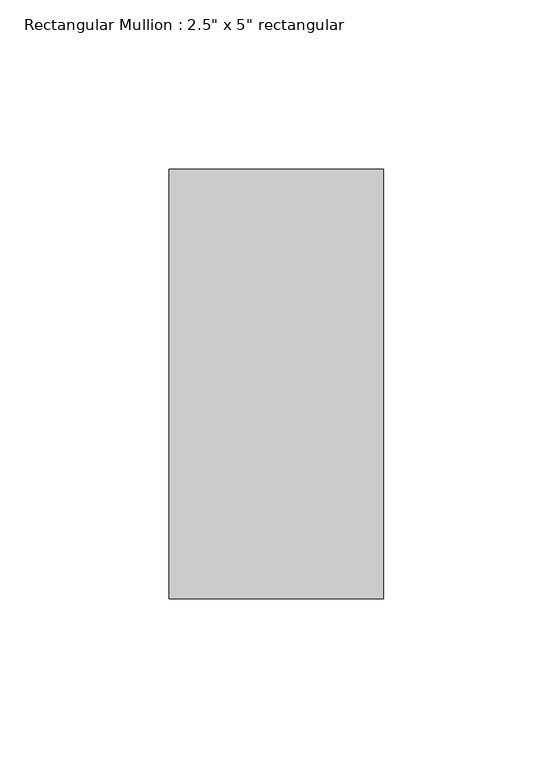
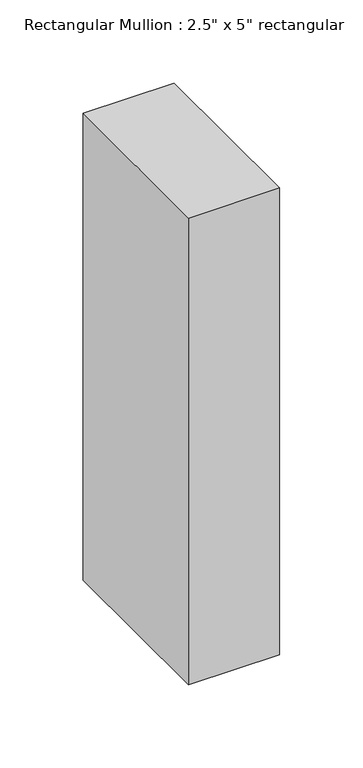
"""IFC4 building model written with IfcOpenShell, lengths in millimetres: member geometry."""

from ifc_helpers import new_model, si_unit, frame, origin, place, context, project, spatial, polyline, outline, extrude, source, transform, mapped, element, save


def member_ff1b7d8f(model_context):
    return source(origin(), model_context, "Body", "SweptSolid", [
        extrude(outline(polyline([(0.0, 63.5), (0.0, -63.5), (-63.5, -63.5), (-63.5, 63.5), (0.0, 63.5)])), frame((0.0, 0.0, -342.9), z_axis=(0.0, 0.0, 1.0), x_axis=(1.0, 0.0, 0.0)), (0.0, 0.0, 1.0), 342.9),
    ])


if __name__ == "__main__":
    model = new_model("IFC4")
    model_context = context("Model", 3, world=origin())
    ifc_project = project(units=[si_unit("LENGTHUNIT", "METRE", prefix="MILLI")], contexts=[model_context])
    site = spatial("IfcSite", under=ifc_project)
    building = spatial("IfcBuilding", under=site)
    placement = place(None, origin())
    member_shape = member_ff1b7d8f(model_context)
    element("IfcMember", 1, ObjectType="Rectangular Mullion : 2.5\" x 5\" rectangular", at=placement, inside=building, context=model_context, shape_type="MappedRepresentation", body=[
        mapped(member_shape, transform((0.0, 0.0, 0.0), x_axis=(1.0, 0.0, 0.0), y_axis=(0.0, 1.0, 0.0), z_axis=(0.0, 0.0, 1.0))),
    ])
    save(model, "model.ifc")

# Revit data of these elements
# Type "Rectangular Mullion : 2.5\" x 5\" rectangular"
#   built-in parameter 1007304 = 0.416667 (stored number, unit not read)
#   built-in parameter 1007301 = 0.104167 (stored number, unit not read)
#   built-in parameter 1007300 = 0.104167 (stored number, unit not read)
# Element 1 (IfcMember, "Rectangular Mullion : 2.5\" x 5\" rectangular")
#   Materials on its faces: "Aluminum"
# Materials
#   "Aluminum": class "Metal", colour RGB 247 247 247, transparency 0, Description = "Aluminum 6061", Cost = 0
